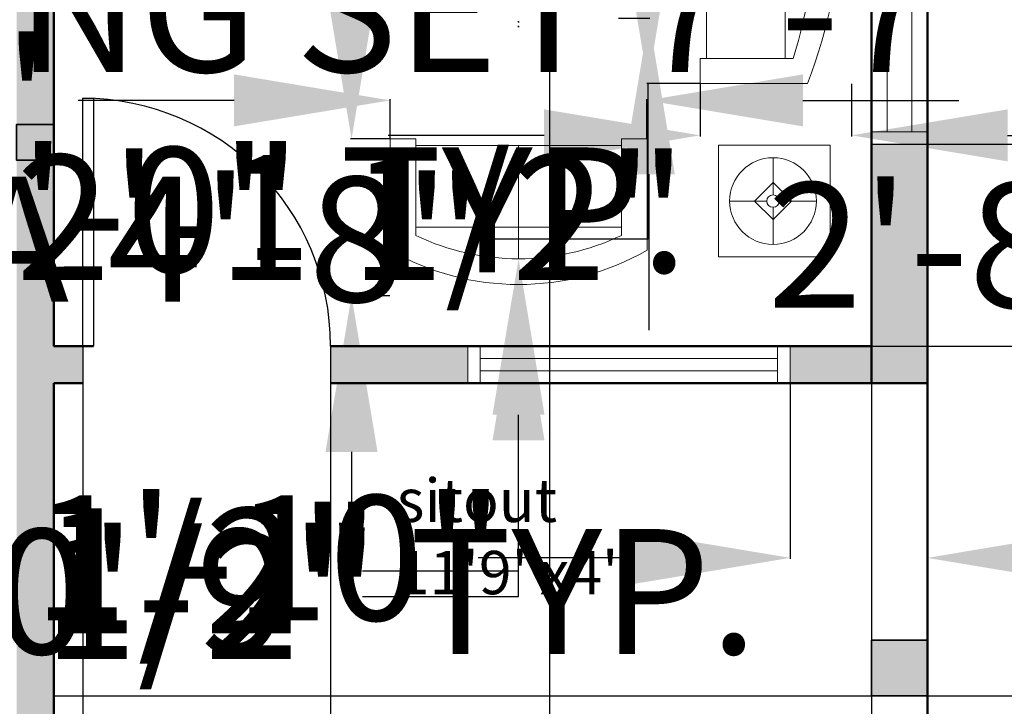
# Model space of a CAD drawing. Units: inches. Extents: x 25 to 82118, y 10 to 6494.
# Tile 5 of 9: x 40928 to 41087, y 3189 to 3300. Entities that reach past the tile are written whole.
import ezdxf

# ---------------------------------------------------------------- set-up
doc = ezdxf.new("R2010")
doc.units = ezdxf.units.IN
doc.header["$MEASUREMENT"] = 0
for name, color, linetype, lineweight in [('A-ANNO-DIMS', 2, 'Continuous', 18), ('A-AREA-IDEN', 7, 'Continuous', 25), ('A-DOOR', 3, 'Continuous', 25), ('A-FLOR-STRS', 7, 'Continuous', 25), ('A-FURN', 8, 'Continuous', 18), ('A-GLAZ', 4, 'Continuous', 18), ('A-WALL', 7, 'Continuous', 50)]:
    doc.layers.add(name, color=color, linetype=linetype, lineweight=lineweight)
doc.layers.add('A-COLS', color=30, linetype='Continuous', lineweight=35, true_color=0xf26722)
doc.layers.add('A-WALL-PATT', color=18, linetype='Continuous', lineweight=13, true_color=0x000000)
doc.styles.get("Standard").update_dxf_attribs({"font": 'arial.ttf'})
doc.dimstyles.get("Standard").update_dxf_attribs({"dimtxt": 20.18, "dimasz": 25.18, "dimexe": 0.18, "dimexo": 0.0625, "dimgap": 0.09, "dimtad": 0, "dimtih": 1, "dimtoh": 1, "dimdec": 0, "dimzin": 0, "dimdsep": 46, "dimlunit": 3, "dimtxsty": 'Standard', "dimcen": 0.09, "dimadec": 0, "dimazin": 0, "dimtfac": 1, "dimtdec": 0, "dimtofl": 0, "dimtmove": 0, "dimatfit": 3, "dimfxl": 1, "dimtolj": 1, "dimtzin": 0, "dimarcsym": 0})

# ---------------------------------------------------------------- blocks, each defined once
blk = doc.blocks.new('Sofa - Roundback 7 ft.')
for p, q in [((-12.00002, -32.4421), (-12.00003, -6.5971)), ((11.99997, -32.4421), (11.99998, -6.5971)), ((-36.000027, -34), (-36.000027, -11.4696)), ((35.99998, -34), (35.99998, -11.4696)), ((-35.999844, -13.3819), (35.9998, -13.3819)), ((-36.000027, -32.4421), (35.99998, -32.4421))]:
    blk.add_line(p, q)
for points in [[(-36.000027, -34), (-42.000027, -34), (-42.000027, -8)], [(41.99998, -8), (41.99998, -34), (35.99998, -34)]]:
    blk.add_lwpolyline(points)
for centre, radius, start, end in [((0, -114.25), 114.25, 68.43141, 111.5686), ((-0.00001, -127.1968), 121.1968, 72.72033, 107.2797)]:
    blk.add_arc(centre, radius, start, end)
blk = doc.blocks.new('*U12')
for p, q in [((0, 0), (0, -6)), ((40, 0), (40, -6))]:
    blk.add_line(p, q)
blk.add_lwpolyline([(0, 0), (0, 40), (1.75, 40), (1.75, 0)], close=True)
blk.add_arc((0, 0), 40, 0, 90)
blk = doc.blocks.new('Lamp - Table')
for p, q in [((0, 7), (0, 1)), ((0, 3), (-3, 0)), ((3, 0), (0, 3)), ((-1, 0), (-7, 0)), ((-3, 0), (0, -3)), ((0, -3), (3, 0)), ((1, 0), (7, 0)), ((0, -1), (0, -7))]:
    blk.add_line(p, q)
for radius in [7, 1]:
    blk.add_circle((0, 0), radius)
blk = doc.blocks.new('Sofa - Roundback Loveseat 5 ft.')
for p, q in [((0, -32.44198), (0, -5.99998)), ((-24, -33.99998), (-24, -11.46958)), ((24.00004, -33.99998), (24.00004, -11.46958)), ((-23.9998, -13.38178), (23.99986, -13.38178)), ((-24, -32.44198), (24.00004, -32.44198))]:
    blk.add_line(p, q)
for points in [[(-24, -33.99998), (-30, -33.99998), (-30, -7.99998)], [(30.00004, -7.99998), (30.00004, -33.99998), (24.00004, -33.99998)]]:
    blk.add_lwpolyline(points)
for centre, radius, start, end in [((0, -60.24998), 60.24998, 60.13715, 119.8628), ((0, -61.38438), 55.38444, 64.32083, 115.6792)]:
    blk.add_arc(centre, radius, start, end)
blk = doc.blocks.new('*D15')
at = {"layer": 'A-ANNO-DIMS', "color": 0, "lineweight": -2, "transparency": 16777216}
for p, q in [((41074.27, 3531.88), (41136.86, 3531.88)), ((41136.68, 3506.7), (41136.68, 3371.51)), ((41136.68, 3215.52), (41136.68, 3350.71)), ((41074.27, 3190.34), (41136.86, 3190.34))]:
    blk.add_line(p, q, dxfattribs=at)
at = {"layer": 'A-ANNO-DIMS', "color": 0, "transparency": 16777216}
for points in [[(41132.48, 3506.7), (41140.87, 3506.7), (41136.68, 3531.88)], [(41132.48, 3215.52), (41140.87, 3215.52), (41136.68, 3190.34)]]:
    blk.add_solid(points, dxfattribs=at)
at = {"layer": 'Defpoints', "color": 0, "transparency": 16777216}
for p in [(41074.21, 3531.88), (41074.21, 3190.34), (41136.68, 3190.34)]:
    blk.add_point(p, dxfattribs=at)
at = {"layer": 'A-ANNO-DIMS', "color": 0, "transparency": 16777216, "insert": (41136.68, 3361.11), "char_height": 20.18, "attachment_point": 5}
blk.add_mtext('\\A1;26\'3"', dxfattribs=at)
blk = doc.blocks.new('*D16')
at = {"layer": 'A-ANNO-DIMS', "color": 0, "lineweight": -2, "transparency": 16777216}
for p, q in [((41074.33, 3531.88), (41191.01, 3531.88)), ((41190.83, 3506.7), (41190.83, 3350.25)), ((41190.83, 3173), (41190.83, 3329.45)), ((41074.33, 3147.82), (41191.01, 3147.82))]:
    blk.add_line(p, q, dxfattribs=at)
at = {"layer": 'A-ANNO-DIMS', "color": 0, "transparency": 16777216}
for points in [[(41186.63, 3506.7), (41195.02, 3506.7), (41190.83, 3531.88)], [(41186.63, 3173), (41195.02, 3173), (41190.83, 3147.82)]]:
    blk.add_solid(points, dxfattribs=at)
at = {"layer": 'Defpoints', "color": 0, "transparency": 16777216}
for p in [(41074.27, 3531.88), (41074.27, 3147.82), (41190.83, 3147.82)]:
    blk.add_point(p, dxfattribs=at)
at = {"layer": 'A-ANNO-DIMS', "color": 0, "transparency": 16777216, "insert": (41190.83, 3339.85), "char_height": 20.18, "attachment_point": 5}
blk.add_mtext("\\A1;32'", dxfattribs=at)
blk = doc.blocks.new('*D17')
at = {"layer": 'A-ANNO-DIMS', "color": 0, "lineweight": -2, "transparency": 16777216}
for p, q in [((41108.65, 3215.52), (41108.65, 3240.7)), ((41074.27, 3190.34), (41108.83, 3190.34)), ((41074.4, 3147.82), (41108.83, 3147.82)), ((41108.65, 3122.64), (41108.65, 3097.46))]:
    blk.add_line(p, q, dxfattribs=at)
at = {"layer": 'A-ANNO-DIMS', "color": 0, "transparency": 16777216}
for points in [[(41104.46, 3215.52), (41112.85, 3215.52), (41108.65, 3190.34)], [(41104.46, 3122.64), (41112.85, 3122.64), (41108.65, 3147.82)]]:
    blk.add_solid(points, dxfattribs=at)
at = {"layer": 'Defpoints', "color": 0, "transparency": 16777216}
for p in [(41074.21, 3190.34), (41074.33, 3147.82), (41108.65, 3147.82)]:
    blk.add_point(p, dxfattribs=at)
at = {"layer": 'A-ANNO-DIMS', "color": 0, "transparency": 16777216, "insert": (41108.65, 3169.08), "char_height": 20.18, "attachment_point": 5}
blk.add_mtext('\\A1;5\'9"', dxfattribs=at)
blk = doc.blocks.new('WIN-72IN-9W')
for p, q in [((9, 76), (0, 76)), ((9, 74), (0, 74)), ((2.5, 74), (2.5, 2)), ((6.5, 74), (6.5, 2)), ((9, 2), (0, 2)), ((9, 0), (0, 0))]:
    blk.add_line(p, q)
blk = doc.blocks.new('COL-9X9')
h = blk.add_hatch(color=256)
h.dxf.hatch_style = 1
h.paths.add_polyline_path([(9, 9), (0, 9), (0, 0), (9, 0)])
blk.add_lwpolyline([(0, 0), (9, 0), (9, 9), (0, 9)], close=True)
blk = doc.blocks.new('POST-INTERIOR-6IN')
h = blk.add_hatch(color=256)
h.dxf.hatch_style = 1
h.paths.add_polyline_path([(6, 5.8), (0, 5.8), (0, 0), (6, 0)])
blk.add_lwpolyline([(6, 5.8), (0, 5.8), (0, 0), (6, 0)], close=True)
blk = doc.blocks.new('*D32')
at = {"layer": 'A-ANNO-DIMS', "color": 0, "lineweight": -2, "transparency": 16777216}
for p, q in [((40898.43, 3182), (40898.43, 3207.18)), ((40898.43, 3207.18), (40923.61, 3207.18)), ((40890.7, 3156.82), (40898.61, 3156.82)), ((40890.7, 3147.82), (40898.61, 3147.82)), ((40898.43, 3122.64), (40898.43, 3097.46))]:
    blk.add_line(p, q, dxfattribs=at)
at = {"layer": 'A-ANNO-DIMS', "color": 0, "transparency": 16777216}
for points in [[(40894.24, 3182), (40902.63, 3182), (40898.43, 3156.82)], [(40894.24, 3122.64), (40902.63, 3122.64), (40898.43, 3147.82)]]:
    blk.add_solid(points, dxfattribs=at)
at = {"layer": 'Defpoints', "color": 0, "transparency": 16777216}
for p in [(40890.63, 3156.82), (40898.43, 3156.82), (40890.63, 3147.82)]:
    blk.add_point(p, dxfattribs=at)
at = {"layer": 'A-ANNO-DIMS', "color": 0, "transparency": 16777216, "insert": (40985.21, 3207.18), "char_height": 20.18, "attachment_point": 5}
blk.add_mtext('\\A1;0\'-9" TYP.', dxfattribs=at)
blk = doc.blocks.new('*D36')
at = {"layer": 'A-ANNO-DIMS', "color": 0, "lineweight": -2, "transparency": 16777216}
for p, q in [((40887.21, 3243.62), (40887.21, 3268.8)), ((40887.21, 3268.8), (40912.39, 3268.8)), ((40875.27, 3243.62), (40887.39, 3243.62)), ((40887.21, 3208.8), (40887.21, 3218.44)), ((40875.27, 3183.62), (40887.39, 3183.62))]:
    blk.add_line(p, q, dxfattribs=at)
at = {"layer": 'A-ANNO-DIMS', "color": 0, "transparency": 16777216}
for points in [[(40883.01, 3218.44), (40891.41, 3218.44), (40887.21, 3243.62)], [(40883.01, 3208.8), (40891.41, 3208.8), (40887.21, 3183.62)]]:
    blk.add_solid(points, dxfattribs=at)
at = {"layer": 'Defpoints', "color": 0, "transparency": 16777216}
for p in [(40875.21, 3243.62), (40887.21, 3243.62), (40875.21, 3183.62)]:
    blk.add_point(p, dxfattribs=at)
at = {"layer": 'A-ANNO-DIMS', "color": 0, "transparency": 16777216, "insert": (40973.98, 3268.8), "char_height": 20.18, "attachment_point": 5}
blk.add_mtext('\\A1;5\'-0" TYP.', dxfattribs=at)
blk = doc.blocks.new('*D43')
at = {"layer": 'A-ANNO-DIMS', "color": 0, "lineweight": -2, "transparency": 16777216}
for p, q in [((41029.25, 3357.91), (41029.25, 3383.09)), ((41024.37, 3332.73), (41029.43, 3332.73)), ((41024.37, 3299.75), (41029.43, 3299.75)), ((41029.25, 3274.57), (41029.25, 3249.39))]:
    blk.add_line(p, q, dxfattribs=at)
at = {"layer": 'A-ANNO-DIMS', "color": 0, "transparency": 16777216}
for points in [[(41025.05, 3357.91), (41033.45, 3357.91), (41029.25, 3332.73)], [(41025.05, 3274.57), (41033.45, 3274.57), (41029.25, 3299.75)]]:
    blk.add_solid(points, dxfattribs=at)
at = {"layer": 'Defpoints', "color": 0, "transparency": 16777216}
for p in [(41024.3, 3332.73), (41029.25, 3332.73), (41024.3, 3299.75)]:
    blk.add_point(p, dxfattribs=at)
at = {"layer": 'A-ANNO-DIMS', "color": 0, "transparency": 16777216, "insert": (41029.25, 3316.24), "char_height": 20.18, "attachment_point": 5}
blk.add_mtext('\\A1;COFFEE TABLE 2\'-9"', dxfattribs=at)
blk = doc.blocks.new('*D45')
at = {"layer": 'A-ANNO-DIMS', "color": 0, "lineweight": -2, "transparency": 16777216}
for p, q in [((41037.46, 3345.25), (41028.94, 3345.25)), ((41029.12, 3320.07), (41029.12, 3314.42)), ((41037.46, 3289.24), (41028.94, 3289.24)), ((41029.12, 3289.24), (41029.12, 3264.06)), ((41029.12, 3264.06), (41003.94, 3264.06))]:
    blk.add_line(p, q, dxfattribs=at)
at = {"layer": 'A-ANNO-DIMS', "color": 0, "transparency": 16777216}
for points in [[(41024.92, 3320.07), (41033.32, 3320.07), (41029.12, 3345.25)], [(41024.92, 3314.42), (41033.32, 3314.42), (41029.12, 3289.24)]]:
    blk.add_solid(points, dxfattribs=at)
at = {"layer": 'Defpoints', "color": 0, "transparency": 16777216}
for p in [(41037.52, 3345.25), (41029.12, 3289.24), (41037.52, 3289.24)]:
    blk.add_point(p, dxfattribs=at)
at = {"layer": 'A-ANNO-DIMS', "color": 0, "transparency": 16777216, "insert": (40934.78, 3264.06), "char_height": 20.18, "attachment_point": 5}
blk.add_mtext('\\A1;SOFA 4\'-8"', dxfattribs=at)
blk = doc.blocks.new('*D46')
at = {"layer": 'A-ANNO-DIMS', "color": 0, "lineweight": -2, "transparency": 16777216}
for p, q in [((41037.52, 3289.18), (41037.52, 3280.66)), ((41061.97, 3289.18), (41061.97, 3280.66)), ((41012.34, 3280.84), (40987.16, 3280.84)), ((41087.15, 3280.84), (41112.33, 3280.84))]:
    blk.add_line(p, q, dxfattribs=at)
at = {"layer": 'A-ANNO-DIMS', "color": 0, "transparency": 16777216}
for points in [[(41012.34, 3285.04), (41012.34, 3276.64), (41037.52, 3280.84)], [(41087.15, 3285.04), (41087.15, 3276.64), (41061.97, 3280.84)]]:
    blk.add_solid(points, dxfattribs=at)
at = {"layer": 'Defpoints', "color": 0, "transparency": 16777216}
for p in [(41037.52, 3289.24), (41061.97, 3289.24), (41061.97, 3280.84)]:
    blk.add_point(p, dxfattribs=at)
at = {"layer": 'A-ANNO-DIMS', "color": 0, "transparency": 16777216, "insert": (41162.92, 3280.84), "char_height": 20.18, "attachment_point": 5}
blk.add_mtext('\\A1;2\'-0 1/2"', dxfattribs=at)
blk = doc.blocks.new('*D47')
at = {"layer": 'A-ANNO-DIMS', "color": 0, "lineweight": -2, "transparency": 16777216}
for p, q in [((40753.09, 3314.74), (40753.09, 3300.97)), ((40844.09, 3314.74), (40844.09, 3300.97)), ((40778.27, 3301.15), (40818.91, 3301.15)), ((40844.09, 3301.15), (40869.27, 3301.15))]:
    blk.add_line(p, q, dxfattribs=at)
at = {"layer": 'A-ANNO-DIMS', "color": 0, "transparency": 16777216}
for points in [[(40778.27, 3305.35), (40778.27, 3296.95), (40753.09, 3301.15)], [(40818.91, 3305.35), (40818.91, 3296.95), (40844.09, 3301.15)]]:
    blk.add_solid(points, dxfattribs=at)
at = {"layer": 'Defpoints', "color": 0, "transparency": 16777216}
for p in [(40753.09, 3314.8), (40844.09, 3314.8), (40844.09, 3301.15)]:
    blk.add_point(p, dxfattribs=at)
at = {"layer": 'A-ANNO-DIMS', "color": 0, "transparency": 16777216, "insert": (40980.26, 3301.15), "char_height": 20.18, "attachment_point": 5}
blk.add_mtext('\\A1;DINING SET 7\'-7"', dxfattribs=at)
blk = doc.blocks.new('*D49')
at = {"layer": 'A-ANNO-DIMS', "color": 0, "lineweight": -2, "transparency": 16777216}
for p, q in [((40987.49, 3280.33), (40987.49, 3286.67)), ((41028.96, 3280.33), (41028.96, 3286.67)), ((40962.31, 3286.49), (40937.13, 3286.49)), ((41054.14, 3286.49), (41079.32, 3286.49))]:
    blk.add_line(p, q, dxfattribs=at)
at = {"layer": 'A-ANNO-DIMS', "color": 0, "transparency": 16777216}
for points in [[(40962.31, 3290.68), (40962.31, 3282.29), (40987.49, 3286.49)], [(41054.14, 3290.68), (41054.14, 3282.29), (41028.96, 3286.49)]]:
    blk.add_solid(points, dxfattribs=at)
at = {"layer": 'Defpoints', "color": 0, "transparency": 16777216}
for p in [(40987.49, 3286.49), (40987.49, 3280.26), (41028.96, 3280.26)]:
    blk.add_point(p, dxfattribs=at)
at = {"layer": 'A-ANNO-DIMS', "color": 0, "transparency": 16777216, "insert": (40808.81, 3286.49), "char_height": 20.18, "attachment_point": 5}
blk.add_mtext('\\A1;LOVESEAT 3\'-5 1/2"', dxfattribs=at)
blk = doc.blocks.new('*D50')
at = {"layer": 'A-ANNO-DIMS', "color": 0, "lineweight": -2, "transparency": 16777216}
for p, q in [((40981.27, 3305.44), (40981.27, 3330.62)), ((40987.43, 3280.26), (40981.09, 3280.26)), ((40987.43, 3254.92), (40981.09, 3254.92)), ((40981.27, 3229.74), (40981.27, 3204.56))]:
    blk.add_line(p, q, dxfattribs=at)
at = {"layer": 'A-ANNO-DIMS', "color": 0, "transparency": 16777216}
for points in [[(40977.07, 3305.44), (40985.46, 3305.44), (40981.27, 3280.26)], [(40977.07, 3229.74), (40985.46, 3229.74), (40981.27, 3254.92)]]:
    blk.add_solid(points, dxfattribs=at)
at = {"layer": 'Defpoints', "color": 0, "transparency": 16777216}
for p in [(40987.49, 3280.26), (40981.27, 3254.92), (40987.49, 3254.92)]:
    blk.add_point(p, dxfattribs=at)
at = {"layer": 'A-ANNO-DIMS', "color": 0, "transparency": 16777216, "insert": (40981.27, 3267.59), "char_height": 20.18, "attachment_point": 5}
blk.add_mtext('\\A1;2\'-1 1/2"', dxfattribs=at)
blk = doc.blocks.new('*D55')
at = {"layer": 'A-ANNO-DIMS', "color": 0, "lineweight": -2, "transparency": 16777216}
for p, q in [((40937.89, 3240.76), (40937.89, 3119.41)), ((40977.89, 3240.76), (40977.89, 3119.41)), ((40912.71, 3119.59), (40887.53, 3119.59)), ((41003.07, 3119.59), (41028.25, 3119.59))]:
    blk.add_line(p, q, dxfattribs=at)
at = {"layer": 'A-ANNO-DIMS', "color": 0, "transparency": 16777216}
for points in [[(40912.71, 3123.78), (40912.71, 3115.39), (40937.89, 3119.59)], [(41003.07, 3123.78), (41003.07, 3115.39), (40977.89, 3119.59)]]:
    blk.add_solid(points, dxfattribs=at)
at = {"layer": 'Defpoints', "color": 0, "transparency": 16777216}
for p in [(40937.89, 3240.82), (40977.89, 3240.82), (40977.89, 3119.59)]:
    blk.add_point(p, dxfattribs=at)
at = {"layer": 'A-ANNO-DIMS', "color": 0, "transparency": 16777216, "insert": (41055.16, 3119.59), "char_height": 20.18, "attachment_point": 5}
blk.add_mtext('\\A1;3\'-4"', dxfattribs=at)
blk = doc.blocks.new('*D65')
at = {"layer": 'A-ANNO-DIMS', "color": 0, "lineweight": -2, "transparency": 16777216}
for p, q in [((41102.56, 3304.59), (41102.56, 3329.77)), ((41065.27, 3279.41), (41102.74, 3279.41)), ((41065.27, 3246.82), (41102.74, 3246.82)), ((41102.56, 3221.64), (41102.56, 3196.46))]:
    blk.add_line(p, q, dxfattribs=at)
at = {"layer": 'A-ANNO-DIMS', "color": 0, "transparency": 16777216}
for points in [[(41098.36, 3304.59), (41106.76, 3304.59), (41102.56, 3279.41)], [(41098.36, 3221.64), (41106.76, 3221.64), (41102.56, 3246.82)]]:
    blk.add_solid(points, dxfattribs=at)
at = {"layer": 'Defpoints', "color": 0, "transparency": 16777216}
for p in [(41065.21, 3279.41), (41102.56, 3279.41), (41065.21, 3246.82)]:
    blk.add_point(p, dxfattribs=at)
at = {"layer": 'A-ANNO-DIMS', "color": 0, "transparency": 16777216, "insert": (41102.56, 3263.11), "char_height": 20.18, "attachment_point": 5}
blk.add_mtext('\\A1;2\'-8 1/2"', dxfattribs=at)
blk = doc.blocks.new('*D66')
at = {"layer": 'A-ANNO-DIMS', "color": 0, "lineweight": -2, "transparency": 16777216}
for p, q in [((41013.21, 3522.76), (41013.21, 3119.41)), ((41065.21, 3522.76), (41065.21, 3119.41)), ((41038.39, 3119.59), (41040.03, 3119.59)), ((41065.21, 3119.59), (41090.39, 3119.59))]:
    blk.add_line(p, q, dxfattribs=at)
at = {"layer": 'A-ANNO-DIMS', "color": 0, "transparency": 16777216}
for points in [[(41038.39, 3123.78), (41038.39, 3115.39), (41013.21, 3119.59)], [(41040.03, 3123.78), (41040.03, 3115.39), (41065.21, 3119.59)]]:
    blk.add_solid(points, dxfattribs=at)
at = {"layer": 'Defpoints', "color": 0, "transparency": 16777216}
for p in [(41013.21, 3522.82), (41065.21, 3522.82), (41065.21, 3119.59)]:
    blk.add_point(p, dxfattribs=at)
at = {"layer": 'A-ANNO-DIMS', "color": 0, "transparency": 16777216, "insert": (41117.71, 3119.59), "char_height": 20.18, "attachment_point": 5}
blk.add_mtext('\\A1;4\'-4"', dxfattribs=at)
blk = doc.blocks.new('*D67')
at = {"layer": 'A-ANNO-DIMS', "color": 0, "lineweight": -2, "transparency": 16777216}
for p, q in [((40770.03, 3572.85), (40744.85, 3572.85)), ((40795.21, 3156.88), (40795.21, 3573.03)), ((40838.63, 3156.88), (40838.63, 3573.03)), ((40863.81, 3572.85), (40888.99, 3572.85))]:
    blk.add_line(p, q, dxfattribs=at)
at = {"layer": 'A-ANNO-DIMS', "color": 0, "transparency": 16777216}
for points in [[(40770.03, 3577.05), (40770.03, 3568.66), (40795.21, 3572.85)], [(40863.81, 3577.05), (40863.81, 3568.66), (40838.63, 3572.85)]]:
    blk.add_solid(points, dxfattribs=at)
at = {"layer": 'Defpoints', "color": 0, "transparency": 16777216}
for p in [(40838.63, 3572.85), (40795.21, 3156.82), (40838.63, 3156.82)]:
    blk.add_point(p, dxfattribs=at)
at = {"layer": 'A-ANNO-DIMS', "color": 0, "transparency": 16777216, "insert": (40939.41, 3572.85), "char_height": 20.18, "attachment_point": 5}
blk.add_mtext('\\A1;3\'-7 1/2"', dxfattribs=at)
blk = doc.blocks.new('*D68')
at = {"layer": 'A-ANNO-DIMS', "color": 0, "lineweight": -2, "transparency": 16777216}
for p, q in [((41052.05, 3240.76), (41052.05, 3212.44)), ((41074.21, 3240.76), (41074.21, 3212.44)), ((41026.87, 3212.62), (41001.69, 3212.62)), ((41099.39, 3212.62), (41124.57, 3212.62))]:
    blk.add_line(p, q, dxfattribs=at)
at = {"layer": 'A-ANNO-DIMS', "color": 0, "transparency": 16777216}
for points in [[(41026.87, 3216.82), (41026.87, 3208.42), (41052.05, 3212.62)], [(41099.39, 3216.82), (41099.39, 3208.42), (41074.21, 3212.62)]]:
    blk.add_solid(points, dxfattribs=at)
at = {"layer": 'Defpoints', "color": 0, "transparency": 16777216}
for p in [(41052.05, 3240.82), (41074.21, 3240.82), (41052.05, 3212.62)]:
    blk.add_point(p, dxfattribs=at)
at = {"layer": 'A-ANNO-DIMS', "color": 0, "transparency": 16777216, "insert": (40967.89, 3212.62), "char_height": 20.18, "attachment_point": 5}
blk.add_mtext('\\A1;1\'-10"', dxfattribs=at)
blk = doc.blocks.new('*D71')
at = {"layer": 'A-ANNO-DIMS', "color": 0, "lineweight": -2, "transparency": 16777216}
for p, q in [((41008.14, 3298.41), (41008.32, 3298.41)), ((41008.23, 3298.32), (41008.23, 3298.5)), ((41008.23, 3206.4), (41008.23, 3231.58)), ((40983.05, 3206.4), (41008.23, 3206.4))]:
    blk.add_line(p, q, dxfattribs=at)
at = {"layer": 'A-ANNO-DIMS', "color": 0, "transparency": 16777216}
blk.add_solid([(41004.03, 3231.58), (41012.42, 3231.58), (41008.23, 3256.76)], dxfattribs=at)
at = {"layer": 'Defpoints', "color": 0, "transparency": 16777216}
for p in [(41008.23, 3298.41), (41008.23, 3256.76)]:
    blk.add_point(p, dxfattribs=at)
at = {"layer": 'A-ANNO-DIMS', "color": 0, "transparency": 16777216, "insert": (40922.97, 3206.4), "char_height": 20.18, "attachment_point": 5}
blk.add_mtext('\\A1;R3\'-5 1/2"', dxfattribs=at)
blk = doc.blocks.new('*D72')
at = {"layer": 'A-ANNO-DIMS', "color": 0, "lineweight": -2, "transparency": 16777216}
for p, q in [((41008.14, 3299.19), (41008.32, 3299.19)), ((41008.23, 3299.1), (41008.23, 3299.28)), ((41008.23, 3210.55), (41008.23, 3235.73)), ((40983.05, 3210.55), (41008.23, 3210.55))]:
    blk.add_line(p, q, dxfattribs=at)
at = {"layer": 'A-ANNO-DIMS', "color": 0, "transparency": 16777216}
blk.add_solid([(41004.03, 3235.73), (41012.42, 3235.73), (41008.23, 3260.91)], dxfattribs=at)
at = {"layer": 'Defpoints', "color": 0, "transparency": 16777216}
for p in [(41008.23, 3299.19), (41008.23, 3260.91)]:
    blk.add_point(p, dxfattribs=at)
at = {"layer": 'A-ANNO-DIMS', "color": 0, "transparency": 16777216, "insert": (40922.97, 3210.55), "char_height": 20.18, "attachment_point": 5}
blk.add_mtext('\\A1;R3\'-2 1/2"', dxfattribs=at)

msp = doc.modelspace()

# ---------------------------------------------------------------- hatches: boundary and pattern name
at = {"layer": 'A-WALL-PATT'}
h = msp.add_hatch(color=256, dxfattribs=at)
h.dxf.hatch_style = 1
h.paths.add_polyline_path([(40778.43, 3531.82), (40723.21, 3531.82), (40723.21, 3522.82), (40778.54, 3522.82, -0.01877), (40778.43, 3525.82)])
h.paths.add_polyline_path([(40723.21, 3522.82), (40714.21, 3522.82), (40714.21, 3500.82), (40723.21, 3500.82)])
h.paths.add_polyline_path([(40723.21, 3424.82), (40714.21, 3424.82), (40714.21, 3404.03), (40723.21, 3404.03)])
h.paths.add_polyline_path([(40723.21, 3395.03), (40714.21, 3395.03), (40714.21, 3386.82), (40723.21, 3386.82)])
h.paths.add_polyline_path([(40901.65, 3531.82), (40834.16, 3531.82), (40834.16, 3522.82), (40901.65, 3522.82)])
h.paths.add_polyline_path([(40825.16, 3531.82), (40818.43, 3531.82), (40818.43, 3525.82), (40818.43, 3522.82), (40825.16, 3522.82)])
h.paths.add_polyline_path([(40961.21, 3531.82), (40910.65, 3531.82), (40910.65, 3522.82), (40961.21, 3522.82)])
h.paths.add_polyline_path([(41065.21, 3531.82), (41013.21, 3531.82), (41013.21, 3522.82), (41065.21, 3522.82)])
h.paths.add_polyline_path([(41074.21, 3522.82), (41065.21, 3522.82), (41065.21, 3506.52), (41074.21, 3506.52)])
h.paths.add_polyline_path([(41074.21, 3430.52), (41065.21, 3430.52), (41065.21, 3428.74), (41065.21, 3380.62), (41074.21, 3380.62)])
h.paths.add_polyline_path([(41074.21, 3371.62), (41065.21, 3371.62), (41065.21, 3355.41), (41074.21, 3355.41)])
h.paths.add_polyline_path([(41065.36, 3378.82), (40909.21, 3378.82), (40909.21, 3382.1), (40903.21, 3382.1), (40903.21, 3372.82), (41065.36, 3372.82)])
h.paths.add_polyline_path([(40933.21, 3372.82), (40927.21, 3372.82), (40927.21, 3282.62), (40933.21, 3282.62)])
h.paths.add_polyline_path([(41074.21, 3279.41), (41065.21, 3279.41), (41065.21, 3240.82), (41074.21, 3240.82)])
h.paths.add_polyline_path([(41065.21, 3246.82), (41052.05, 3246.82), (41052.05, 3240.82), (41065.21, 3240.82)])
h.paths.add_polyline_path([(40985.75, 3202.89), (41023.1, 3202.89), (41023.1, 3229.01), (40985.75, 3229.01)], flags=9)
h.paths.add_polyline_path([(40960.75, 3302.54), (40998.1, 3302.54), (40998.1, 3328.66), (40960.75, 3328.66)], flags=9)
h = msp.add_hatch(color=256, dxfattribs=at)
h.dxf.hatch_style = 1
h.paths.add_polyline_path([(40723.21, 3274), (40714.21, 3274), (40714.21, 3212.82), (40723.21, 3212.82), (40723.21, 3240.82), (40760.88, 3240.82, -0.030698), (40760.71, 3243.52), (40760.71, 3246.82), (40723.21, 3246.82)])
h.paths.add_polyline_path([(40789.21, 3246.82), (40782.73, 3246.82), (40782.73, 3243.52), (40782.73, 3240.82), (40789.21, 3240.82)])
h.paths.add_polyline_path([(40795.21, 3276.82), (40880.67, 3276.82), (40880.67, 3282.82), (40789.21, 3282.82), (40789.21, 3240.82), (40795.21, 3240.82), (40795.21, 3243.62)])
h.paths.add_polyline_path([(40795.21, 3240.82), (40789.21, 3240.82), (40789.21, 3156.82), (40723.21, 3156.82), (40723.21, 3147.82), (40838.63, 3147.82), (40838.63, 3156.82), (40795.21, 3156.82)])
h.paths.add_polyline_path([(40723.21, 3184.82), (40714.21, 3184.82), (40714.21, 3156.79), (40723.21, 3156.79), (40723.21, 3156.82)])
h.paths.add_polyline_path([(40924.06, 3156.82), (40890.63, 3156.82), (40890.63, 3147.82), (40924.06, 3147.82)])
h.paths.add_polyline_path([(40933.21, 3240.82), (40937.89, 3240.82), (40937.89, 3246.82), (40933.21, 3246.82), (40933.21, 3276.82), (40927.21, 3276.82), (40927.21, 3156.82), (40933.21, 3156.82)])
h.paths.add_polyline_path([(41000.05, 3246.82), (40977.89, 3246.82), (40977.89, 3240.82), (41000.05, 3240.82)])

# ---------------------------------------------------------------- linework, layer by layer
at = {"layer": 'A-FLOR-STRS'}
msp.add_line((40933.21, 3190.34), (41074.21, 3190.34), dxfattribs=at)
at = {"layer": 'A-FURN'}
msp.add_lwpolyline([(41040.49, 3279.24), (41058.54, 3279.24), (41058.54, 3261.21), (41040.49, 3261.21)], close=True, dxfattribs=at)
at = {"layer": 'A-GLAZ'}
for p, q in [((41000.05, 3240.82), (41000.05, 3246.82)), ((41002.05, 3240.82), (41002.05, 3246.82)), ((41050.05, 3240.82), (41050.05, 3246.82)), ((41052.05, 3240.82), (41052.05, 3246.82)), ((41002.05, 3244.82), (41050.05, 3244.82)), ((41002.05, 3242.82), (41050.05, 3242.82))]:
    msp.add_line(p, q, dxfattribs=at)
at = {"layer": 'A-WALL'}
for p, q in [((41074.21, 3531.82), (41074.21, 3147.82)), ((40933.21, 3372.82), (40933.21, 3246.82)), ((41065.21, 3372.82), (41065.21, 3240.82)), ((40939.64, 3246.82), (40933.21, 3246.82)), ((41065.21, 3246.82), (40977.89, 3246.82)), ((40933.21, 3240.82), (40933.21, 3147.82)), ((40937.89, 3240.82), (40933.21, 3240.82)), ((41074.21, 3240.82), (40977.89, 3240.82))]:
    msp.add_line(p, q, dxfattribs=at)

# ---------------------------------------------------------------- block references
at = {"layer": 'A-COLS'}
for name, p in [('POST-INTERIOR-6IN', (40927.21, 3276.82)), ('COL-9X9', (41065.21, 3190.34))]:
    msp.add_blockref(name, p, dxfattribs=at)
at = {"layer": 'A-DOOR'}
msp.add_blockref('*U12', (40937.89, 3246.82), dxfattribs=at)
at = {"layer": 'A-FURN'}
for name, p, xscale, yscale, zscale, rotation in [('Sofa - Roundback 7 ft.', (41060.19, 3317.24), 0.666763508743389, 0.666763508743389, 0.666763508743389, 270), ('Sofa - Roundback Loveseat 5 ft.', (41008.23, 3256.76), 0.691284907331284, 0.691284907331284, 0.691284907331284, 180)]:
    msp.add_blockref(name, p, dxfattribs=dict(at, xscale=xscale, yscale=yscale, zscale=zscale, rotation=rotation))
msp.add_blockref('Lamp - Table', (41049.3, 3270.23), dxfattribs=at)
at = {"layer": 'A-GLAZ'}
msp.add_blockref('WIN-72IN-9W', (41065.21, 3279.41), dxfattribs=at)

# ---------------------------------------------------------------- texts
at = {"layer": 'A-AREA-IDEN', "insert": (40988.56, 3225.41), "char_height": 7, "attachment_point": 1}
msp.add_mtext_dynamic_manual_height_columns('sitout\\P11\'9"x4\'', width=132.9687, gutter_width=1, heights=[0], dxfattribs=at)

# ---------------------------------------------------------------- dimensions: what is measured, and where the dimension line sits
at = {"layer": 'A-ANNO-DIMS'}
for base, p1, p2, picture, middle in [((40838.63, 3572.85), (40795.21, 3156.82), (40838.63, 3156.82), '*D67', (40939.41, 3572.85)), ((41065.21, 3119.59), (41013.21, 3522.82), (41065.21, 3522.82), '*D66', (41117.71, 3119.59)), ((41061.9692, 3280.8387), (41037.5212, 3289.2399), (41061.9692, 3289.2399), '*D46', (41162.9243, 3280.8387)), ((40977.89, 3119.59), (40937.89, 3240.82), (40977.89, 3240.82), '*D55', (41055.16, 3119.59))]:
    dim = msp.add_linear_dim(base=base, p1=p1, p2=p2, dimstyle='Standard', override={"dimdec": 1, "dimlfac": 1, "dimrnd": 0, "dimzin": 1, "dimdsep": 46, "dimlunit": 4, "dimfrac": 2}, dxfattribs=at)
    dim.commit()
    dim.dimension.update_dxf_attribs({"geometry": picture, "text_midpoint": middle})
for base, p1, p2, angle, text, override, picture, middle in [((41136.68, 3190.34), (41074.21, 3531.88), (41074.21, 3190.34), 90, '26\'3"', {"dimclrd": 0, "dimclre": 0, "dimclrt": 0}, '*D15', (41136.68, 3361.11)), ((41029.25, 3332.73), (41024.3, 3299.75), (41024.3, 3332.73), 90, 'COFFEE TABLE <>', {"dimdec": 1, "dimlfac": 1, "dimrnd": 0, "dimzin": 1, "dimdsep": 46, "dimlunit": 4, "dimfrac": 2}, '*D43', (41029.25, 3316.24)), ((41029.12, 3289.24), (41037.52, 3345.25), (41037.52, 3289.24), 270, 'SOFA <>', {"dimdec": 1, "dimlfac": 1, "dimrnd": 0, "dimzin": 1, "dimdsep": 46, "dimlunit": 4, "dimfrac": 2}, '*D45', (40934.78, 3264.06)), ((40987.49, 3286.49), (41028.96, 3280.26), (40987.49, 3280.26), 180, 'LOVESEAT <>', {"dimdec": 1, "dimlfac": 1, "dimrnd": 0, "dimzin": 1, "dimdsep": 46, "dimlunit": 4, "dimfrac": 2}, '*D49', (40808.81, 3286.49)), ((40887.21, 3243.62), (40875.21, 3183.62), (40875.21, 3243.62), 90, '<> TYP.', {"dimdec": 1, "dimlfac": 1, "dimrnd": 0, "dimzin": 1, "dimdsep": 46, "dimlunit": 4, "dimfrac": 2}, '*D36', (40973.98, 3268.8)), ((41108.65, 3147.82), (41074.21, 3190.34), (41074.33, 3147.82), 90, '5\'9"', {"dimclrd": 0, "dimclre": 0, "dimclrt": 0}, '*D17', (41108.65, 3169.08)), ((40898.43, 3156.82), (40890.63, 3147.82), (40890.63, 3156.82), 90, '<> TYP.', {"dimdec": 1, "dimlfac": 1, "dimrnd": 0, "dimzin": 1, "dimdsep": 46, "dimlunit": 4, "dimfrac": 2}, '*D32', (40985.21, 3207.18))]:
    dim = msp.add_linear_dim(base=base, p1=p1, p2=p2, angle=angle, text=text, dimstyle='Standard', override=override, dxfattribs=at)
    dim.commit()
    dim.dimension.update_dxf_attribs({"geometry": picture, "text_midpoint": middle})
for base, p1, p2, angle, override, picture, middle in [((41190.83, 3147.82), (41074.27, 3531.88), (41074.27, 3147.82), 90, {"dimclrd": 0, "dimclre": 0, "dimclrt": 0}, '*D16', (41190.83, 3339.85)), ((40981.27, 3254.92), (40987.49, 3280.26), (40987.49, 3254.92), 270, {"dimdec": 1, "dimlfac": 1, "dimrnd": 0, "dimzin": 1, "dimdsep": 46, "dimlunit": 4, "dimfrac": 2}, '*D50', (40981.27, 3267.59)), ((41102.56, 3279.41), (41065.21, 3246.82), (41065.21, 3279.41), 90, {"dimdec": 1, "dimlfac": 1, "dimrnd": 0, "dimzin": 1, "dimdsep": 46, "dimlunit": 4, "dimfrac": 2}, '*D65', (41102.56, 3263.11)), ((41052.05, 3212.62), (41074.21, 3240.82), (41052.05, 3240.82), 180, {"dimdec": 1, "dimlfac": 1, "dimrnd": 0, "dimzin": 1, "dimdsep": 46, "dimlunit": 4, "dimfrac": 2}, '*D68', (40967.89, 3212.62))]:
    dim = msp.add_linear_dim(base=base, p1=p1, p2=p2, angle=angle, dimstyle='Standard', override=override, dxfattribs=at)
    dim.commit()
    dim.dimension.update_dxf_attribs({"geometry": picture, "text_midpoint": middle})
dim = msp.add_linear_dim(base=(40844.09, 3301.15), p1=(40753.09, 3314.8), p2=(40844.09, 3314.8), text='DINING SET <>', dimstyle='Standard', override={"dimdec": 1, "dimlfac": 1, "dimrnd": 0, "dimzin": 1, "dimdsep": 46, "dimlunit": 4, "dimfrac": 2}, dxfattribs=at)
dim.commit()
dim.dimension.update_dxf_attribs({"geometry": '*D47', "text_midpoint": (40980.26, 3301.15)})
for center, mpoint, picture, middle in [((41008.23, 3299.19), (41008.23, 3260.91), '*D72', (40922.97, 3210.55)), ((41008.2264, 3298.4101), (41008.226, 3256.7602), '*D71', (40922.9662, 3206.4002))]:
    dim = msp.add_radius_dim(center=center, mpoint=mpoint, dimstyle='Standard', override={"dimdec": 1, "dimlfac": 1, "dimrnd": 0, "dimzin": 1, "dimdsep": 46, "dimlunit": 4, "dimfrac": 2}, dxfattribs=at)
    dim.commit()
    dim.dimension.update_dxf_attribs({"geometry": picture, "text_midpoint": middle})

doc.saveas('drawing.dxf')
